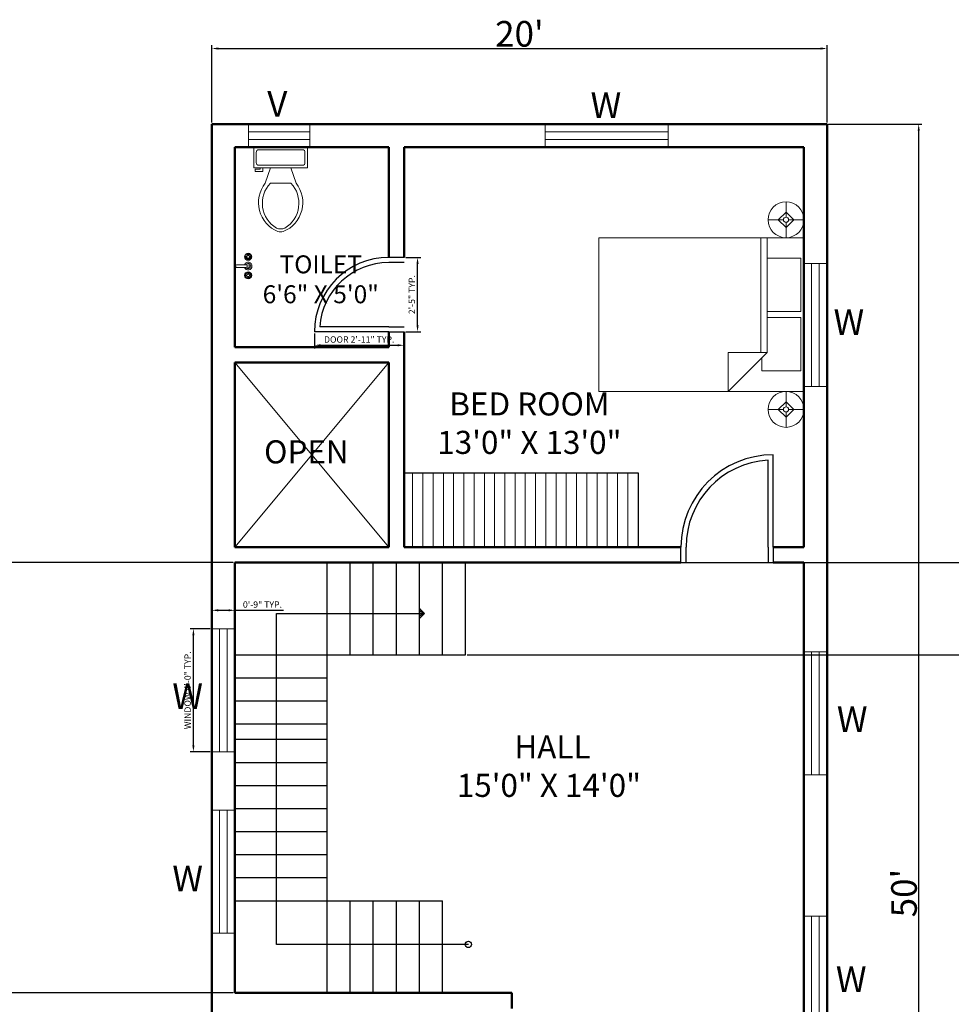
# Model space of a CAD drawing. Units: inches. Extents: x 995 to 2141, y 2161 to 2928.
# Tile 5 of 7: x 1358 to 1721, y 2537 to 2921. Entities that reach past the tile are written whole.
import ezdxf

# ---------------------------------------------------------------- set-up
doc = ezdxf.new("R2010")
doc.units = ezdxf.units.IN
for name, color, linetype, lineweight in [('A-ANNO-DIMS', 2, 'Continuous', 18), ('A-ANNO-TEXT', 7, 'Continuous', 18), ('A-AREA-IDEN', 7, 'Continuous', 25), ('A-DOOR', 3, 'Continuous', 25), ('A-FLOR-CASE', 8, 'Continuous', 25), ('A-FLOR-CASE-PATT', 252, 'Continuous', 13), ('A-FLOR-FIXT', 9, 'Continuous', 18), ('A-FLOR-OPEN', 8, 'Continuous', 13), ('A-FLOR-STRS', 7, 'Continuous', 25), ('A-FURN', 8, 'Continuous', 18), ('A-GLAZ', 4, 'Continuous', 18), ('A-WALL', 7, 'Continuous', 50)]:
    doc.layers.add(name, color=color, linetype=linetype, lineweight=lineweight)
doc.styles.get("Standard").update_dxf_attribs({"font": 'arial.ttf'})
doc.dimstyles.new('ISO-25', dxfattribs={"dimtxt": 2.5, "dimasz": 2.5, "dimexe": 1.25, "dimexo": 0.625, "dimtad": 1, "dimdec": 0, "dimlunit": 3, "dimtxsty": 'Standard', "dimcen": 2.5, "dimadec": 0, "dimazin": 0, "dimtfac": 1, "dimtdec": 0, "dimtmove": 0, "dimatfit": 3, "dimfxl": 1, "dimarcsym": 0})

# ---------------------------------------------------------------- blocks, each defined once
blk = doc.blocks.new('Bed - Queen')
for p, q in [((0, -80.00003), (0, 0)), ((0, 0), (59.99999, 0)), ((59.99999, 0), (59.99999, -80.00003)), ((7.99999, -1.2), (28.79998, -1.2)), ((7.99999, -14.4), (7.99999, -1.2)), ((28.79998, -1.2), (28.79998, -14.4)), ((31.19999, -1.2), (51.99999, -1.2)), ((31.19999, -14.4), (31.19999, -1.2)), ((51.99999, -1.2), (51.99999, -16.4)), ((0, -14.4), (44.8, -14.4)), ((59.99999, -29.6), (44.8, -14.4)), ((44.8, -14.4), (44.8, -29.6)), ((44.8, -16.8), (0, -16.8)), ((51.99999, -16.4), (46.79936, -16.4)), ((44.8, -29.6), (59.99999, -29.6)), ((59.99999, -80.00003), (0, -80.00003))]:
    blk.add_line(p, q)
blk = doc.blocks.new('Lamp - Table')
for p, q in [((0, 7), (0, 1)), ((-1, 0), (-7, 0)), ((0, 3), (-3, 0)), ((-3, 0), (0, -3)), ((3, 0), (0, 3)), ((0, -3), (3, 0)), ((1, 0), (7, 0)), ((0, -1), (0, -7))]:
    blk.add_line(p, q)
for radius in [7, 1]:
    blk.add_circle((0, 0), radius)
blk = doc.blocks.new('Toilet - top')
for p, q in [((9.5, -6), (9.5, -2)), ((-10, -8.5), (-8, -8.5)), ((-10, -9.5), (-10, -8.5)), ((-7, -9.5), (-10, -9.5)), ((-8, -8.5), (-8, -8)), ((-7, -8), (-7, -9.5)), ((-4, -8), (-6, -14)), ((4, -8), (6, -14)), ((4, -14), (-4, -14))]:
    blk.add_line(p, q)
blk.add_lwpolyline([(10.5, -8), (10.5, 0), (-10.5, 0), (-10.5, -8)], close=True)
for points in [[(-9.5, -2), (-9.5, -6)], [(8.5, -1), (-8.5, -1)], [(-8.5, -7), (8.5, -7)]]:
    blk.add_lwpolyline(points)
for centre, radius, start, end in [((-8.62, -1.88), 0.884, 81.8699, 188.1301), ((8.62, -1.88), 0.884, 351.8699, 98.1301), ((-8.62, -6.12), 0.884, 171.8699, 278.1301), ((8.62, -6.12), 0.884, 261.8699, 8.1301), ((3.52, -21.58), 12.17, 141.4691, 247.9714), ((4.2, -21.82), 11.33, 136.3677, 238.9468), ((-3.52, -21.58), 12.17, 292.0284, 38.5307), ((-4.2, -21.82), 11.33, 301.053, 43.6321), ((0, -27.88), 4, 245.7318, 294.2682), ((0, -29), 4, 254.8605, 285.1395)]:
    blk.add_arc(centre, radius, start, end)
blk = doc.blocks.new('Faucet - Bathroom top')
for p, q in [((-4.107, 0.125), (-4.375, 0.125)), ((-3.75, 0.4788), (-3.75, 0.75)), ((-3.5, 0.482), (-3.5, 0.75)), ((-3.1461, 0.125), (-2.875, 0.125)), ((3.143, 0.125), (2.875, 0.125)), ((3.5, 0.4788), (3.5, 0.75)), ((3.75, 0.482), (3.75, 0.75)), ((4.1039, 0.125), (4.375, 0.125)), ((-4.1039, -0.125), (-4.375, -0.125)), ((-3.75, -0.4821), (-3.75, -0.75)), ((-3.5, -0.4789), (-3.5, -0.75)), ((-3.143, -0.125), (-2.875, -0.125)), ((-0.5, -0.8639), (-0.5, -4.5)), ((0.5, -4.5), (0.5, -0.8631)), ((3.1461, -0.125), (2.875, -0.125)), ((3.5, -0.4821), (3.5, -0.75)), ((3.75, -0.4789), (3.75, -0.75)), ((4.107, -0.125), (4.375, -0.125))]:
    blk.add_line(p, q)
for centre, radius in [((-3.625, 0), 1.375), ((-4.625, 0), 0.2795), ((-3.625, 0), 0.5), ((-3.625, 1), 0.2795), ((-2.625, 0), 0.2795), ((0, 0), 0.5), ((3.625, 0), 1.375), ((2.625, 0), 0.2795), ((3.625, 0), 0.5), ((3.625, 1), 0.2795), ((4.625, 0), 0.2795), ((-3.625, -1), 0.2795), ((3.625, -1), 0.2795)]:
    blk.add_circle(centre, radius)
for centre, radius, start, end in [((-3.625, 0), 1, 105.2407, 164.2093), ((-3.625, 0), 1, 16.44125, 74.07887), ((0, 0), 1.5, 289.6514, 250.3603), ((0, 0), 1, 300.3431, 239.7554), ((3.625, 0), 1, 106.12, 164.0884), ((3.625, 0), 1, 16.23422, 73.90469), ((-3.625, 0), 1, 196.2342, 253.9047), ((-3.625, 0), 1, 286.12, 344.0884), ((3.625, 0), 1, 196.4413, 254.0789), ((3.625, 0), 1, 285.2407, 344.2093), ((0, -4.5), 0.5, 180, 0)]:
    blk.add_arc(centre, radius, start, end)
blk = doc.blocks.new('*D18')
at = {"layer": 'A-ANNO-DIMS', "color": 0, "lineweight": -2, "transparency": 16777216}
for p, q in [((1433, 2881.14), (1433, 2911.31)), ((1435.5, 2910.06), (1670.5, 2910.06)), ((1673, 2881.14), (1673, 2911.31))]:
    blk.add_line(p, q, dxfattribs=at)
at = {"layer": 'A-ANNO-DIMS', "color": 0, "transparency": 16777216}
for points in [[(1435.5, 2910.48), (1435.5, 2909.64), (1433, 2910.06)], [(1670.5, 2910.48), (1670.5, 2909.64), (1673, 2910.06)]]:
    blk.add_solid(points, dxfattribs=at)
at = {"layer": 'Defpoints', "color": 0, "transparency": 16777216}
for p in [(1673, 2910.06), (1433, 2880.52), (1673, 2880.52)]:
    blk.add_point(p, dxfattribs=at)
at = {"layer": 'A-ANNO-DIMS', "color": 0, "transparency": 16777216, "insert": (1553, 2915.79), "char_height": 2.5, "attachment_point": 5}
blk.add_mtext("{\\H4x;20'}", dxfattribs=at)
blk = doc.blocks.new('*D21')
at = {"layer": 'A-ANNO-DIMS', "color": 0, "lineweight": -2, "transparency": 16777216}
for p, q in [((1673.63, 2880.52), (1710.02, 2880.52)), ((1708.77, 2283.02), (1708.77, 2878.02)), ((1673.63, 2280.52), (1710.02, 2280.52))]:
    blk.add_line(p, q, dxfattribs=at)
at = {"layer": 'A-ANNO-DIMS', "color": 0, "transparency": 16777216}
for points in [[(1708.36, 2878.02), (1709.19, 2878.02), (1708.77, 2880.52)], [(1708.36, 2283.02), (1709.19, 2283.02), (1708.77, 2280.52)]]:
    blk.add_solid(points, dxfattribs=at)
at = {"layer": 'Defpoints', "color": 0, "transparency": 16777216}
for p in [(1673, 2880.52), (1708.77, 2880.52), (1673, 2280.52)]:
    blk.add_point(p, dxfattribs=at)
at = {"layer": 'A-ANNO-DIMS', "color": 0, "transparency": 16777216, "insert": (1703.04, 2580.52), "char_height": 2.5, "attachment_point": 5, "rotation": 90}
blk.add_mtext("{\\H4x;50'}", dxfattribs=at)
blk = doc.blocks.new('WIN-48IN')
for p, q in [((0, 48), (0, 0)), ((9, 48), (0, 48)), ((3, 48), (3, 0)), ((6, 0), (6, 48)), ((9, 0), (9, 48)), ((0, 0), (9, 0))]:
    blk.add_line(p, q)
blk = doc.blocks.new('VENT-24IN')
for p, q in [((24, 9), (0, 9)), ((0, 9), (0, 0)), ((24, 9), (24, 0)), ((24, 6), (0, 6)), ((0, 3), (24, 3)), ((0, 0), (24, 0))]:
    blk.add_line(p, q)
blk = doc.blocks.new('DOOR-29IN-6IN-JAMB')
for p, q in [((35, 29), (29, 29)), ((35, 27), (29, 27)), ((29, 0), (0, 0)), ((29, 2), (2.07, 2)), ((29, 2), (35, 2)), ((29, 0), (35, 0))]:
    blk.add_line(p, q)
for radius, end in [(29, 180), (27, 175.752)]:
    blk.add_arc((29, 0), radius, 90, end)
blk = doc.blocks.new('DOOR-36IN-SWING')
for p, q in [((36, 0), (36, 36)), ((34, 0), (34, 33.94))]:
    blk.add_line(p, q)
for radius, start in [(36, 90), (34, 93.3723)]:
    blk.add_arc((36, 0), radius, start, 180)
blk = doc.blocks.new('OPENING-CROSS-60X72')
for p, q in [((60, 72), (0, 0)), ((0, 72), (60, 0))]:
    blk.add_line(p, q)
blk = doc.blocks.new('*D28')
at = {"layer": 'A-ANNO-DIMS', "color": 0, "lineweight": -2, "transparency": 16777216}
for p, q in [((1432.38, 2683.64), (1424.55, 2683.64)), ((1425.8, 2638.14), (1425.8, 2681.14)), ((1432.38, 2635.64), (1424.55, 2635.64))]:
    blk.add_line(p, q, dxfattribs=at)
at = {"layer": 'A-ANNO-DIMS', "color": 0, "transparency": 16777216}
for points in [[(1425.39, 2681.14), (1426.22, 2681.14), (1425.8, 2683.64)], [(1425.39, 2638.14), (1426.22, 2638.14), (1425.8, 2635.64)]]:
    blk.add_solid(points, dxfattribs=at)
at = {"layer": 'Defpoints', "color": 0, "transparency": 16777216}
for p in [(1425.8, 2683.64), (1433, 2683.64), (1433, 2635.64)]:
    blk.add_point(p, dxfattribs=at)
at = {"layer": 'A-ANNO-DIMS', "color": 0, "transparency": 16777216, "insert": (1423.88, 2659.64), "char_height": 2.5, "attachment_point": 5, "rotation": 90}
blk.add_mtext('WINDOW 4\'-0" TYP.', dxfattribs=at)
blk = doc.blocks.new('*D29')
at = {"layer": 'A-ANNO-DIMS', "color": 0, "lineweight": -2, "transparency": 16777216}
for p, q in [((1433, 2684.27), (1433, 2692.09)), ((1435.5, 2690.84), (1439.5, 2690.84)), ((1442, 2684.27), (1442, 2692.09)), ((1442, 2690.84), (1460.99, 2690.84))]:
    blk.add_line(p, q, dxfattribs=at)
at = {"layer": 'A-ANNO-DIMS', "color": 0, "transparency": 16777216}
for points in [[(1435.5, 2691.26), (1435.5, 2690.43), (1433, 2690.84)], [(1439.5, 2691.26), (1439.5, 2690.43), (1442, 2690.84)]]:
    blk.add_solid(points, dxfattribs=at)
at = {"layer": 'Defpoints', "color": 0, "transparency": 16777216}
for p in [(1442, 2690.84), (1433, 2683.64), (1442, 2683.64)]:
    blk.add_point(p, dxfattribs=at)
at = {"layer": 'A-ANNO-DIMS', "color": 0, "transparency": 16777216, "insert": (1452.75, 2692.75), "char_height": 2.5, "attachment_point": 5}
blk.add_mtext('0\'-9" TYP.', dxfattribs=at)
blk = doc.blocks.new('*D36')
at = {"layer": 'A-ANNO-DIMS', "color": 0, "lineweight": -2, "transparency": 16777216}
for p, q in [((1473, 2798.89), (1473, 2793.02)), ((1508, 2798.89), (1508, 2793.02)), ((1475.5, 2794.27), (1505.5, 2794.27))]:
    blk.add_line(p, q, dxfattribs=at)
at = {"layer": 'A-ANNO-DIMS', "color": 0, "transparency": 16777216}
for points in [[(1475.5, 2794.68), (1475.5, 2793.85), (1473, 2794.27)], [(1505.5, 2794.68), (1505.5, 2793.85), (1508, 2794.27)]]:
    blk.add_solid(points, dxfattribs=at)
at = {"layer": 'Defpoints', "color": 0, "transparency": 16777216}
for p in [(1473, 2799.52), (1508, 2799.52), (1508, 2794.27)]:
    blk.add_point(p, dxfattribs=at)
at = {"layer": 'A-ANNO-DIMS', "color": 0, "transparency": 16777216, "insert": (1490.5, 2796.19), "char_height": 2.5, "attachment_point": 5}
blk.add_mtext('DOOR 2\'-11" TYP.', dxfattribs=at)
blk = doc.blocks.new('*D37')
at = {"layer": 'A-ANNO-DIMS', "color": 0, "lineweight": -2, "transparency": 16777216}
for p, q in [((1508.63, 2828.52), (1514.5, 2828.52)), ((1513.25, 2802.02), (1513.25, 2826.02)), ((1508.63, 2799.52), (1514.5, 2799.52))]:
    blk.add_line(p, q, dxfattribs=at)
at = {"layer": 'A-ANNO-DIMS', "color": 0, "transparency": 16777216}
for points in [[(1512.84, 2826.02), (1513.67, 2826.02), (1513.25, 2828.52)], [(1512.84, 2802.02), (1513.67, 2802.02), (1513.25, 2799.52)]]:
    blk.add_solid(points, dxfattribs=at)
at = {"layer": 'Defpoints', "color": 0, "transparency": 16777216}
for p in [(1508, 2828.52), (1513.25, 2828.52), (1508, 2799.52)]:
    blk.add_point(p, dxfattribs=at)
at = {"layer": 'A-ANNO-DIMS', "color": 0, "transparency": 16777216, "insert": (1511.35, 2814.02), "char_height": 2.5, "attachment_point": 5, "rotation": 90}
blk.add_mtext('2\'-5" TYP.', dxfattribs=at)
blk = doc.blocks.new('*D64')
at = {"layer": 'A-ANNO-DIMS', "color": 0, "lineweight": -2, "transparency": 16777216}
for p, q in [((1532.63, 2709.52), (2141.3, 2709.52)), ((2140.05, 2676.02), (2140.05, 2707.02)), ((1532.63, 2673.52), (2141.3, 2673.52))]:
    blk.add_line(p, q, dxfattribs=at)
at = {"layer": 'A-ANNO-DIMS', "color": 0, "transparency": 16777216}
for points in [[(2139.63, 2707.02), (2140.46, 2707.02), (2140.05, 2709.52)], [(2139.63, 2676.02), (2140.46, 2676.02), (2140.05, 2673.52)]]:
    blk.add_solid(points, dxfattribs=at)
at = {"layer": 'Defpoints', "color": 0, "transparency": 16777216}
for p in [(1532, 2709.52), (2140.05, 2709.52), (1532, 2673.52)]:
    blk.add_point(p, dxfattribs=at)
at = {"layer": 'A-ANNO-DIMS', "color": 0, "transparency": 16777216, "insert": (2138.14, 2691.52), "char_height": 2.5, "attachment_point": 5, "rotation": 90}
blk.add_mtext('3\'-0"', dxfattribs=at)
blk = doc.blocks.new('*D65')
at = {"layer": 'A-ANNO-DIMS', "color": 0, "lineweight": -2, "transparency": 16777216}
for p, q in [((1441.38, 2709.52), (996.93, 2709.52)), ((998.18, 2544.02), (998.18, 2707.02)), ((1441.38, 2541.52), (996.93, 2541.52))]:
    blk.add_line(p, q, dxfattribs=at)
at = {"layer": 'A-ANNO-DIMS', "color": 0, "transparency": 16777216}
for points in [[(997.77, 2707.02), (998.6, 2707.02), (998.18, 2709.52)], [(997.77, 2544.02), (998.6, 2544.02), (998.18, 2541.52)]]:
    blk.add_solid(points, dxfattribs=at)
at = {"layer": 'Defpoints', "color": 0, "transparency": 16777216}
for p in [(998.18, 2709.52), (1442, 2709.52), (1442, 2541.52)]:
    blk.add_point(p, dxfattribs=at)
at = {"layer": 'A-ANNO-DIMS', "color": 0, "transparency": 16777216, "insert": (996.28, 2625.52), "char_height": 2.5, "attachment_point": 5, "rotation": 90}
blk.add_mtext('14\'-0"', dxfattribs=at)

msp = doc.modelspace()

# ---------------------------------------------------------------- hatches: boundary and pattern name
at = {"layer": 'A-FLOR-CASE-PATT'}
h = msp.add_hatch(dxfattribs=at)
h.set_pattern_fill('ANSI31', color=256, scale=1.259274, angle=45, style=0)
h.paths.add_polyline_path([(1509.3, 2715.52), (1597.3, 2715.52), (1597.3, 2744.52), (1509.3, 2744.52)])

# ---------------------------------------------------------------- linework, layer by layer
at = {"layer": 'A-DOOR'}
for p, q in [((1616, 2709.52), (1616, 2715.52)), ((1618, 2709.52), (1618, 2715.52)), ((1650, 2715.52), (1650, 2709.52)), ((1652, 2715.52), (1652, 2709.52))]:
    msp.add_line(p, q, dxfattribs=at)
at = {"layer": 'A-FLOR-CASE'}
for p, q in [((1508, 2744.52), (1599.3, 2744.52)), ((1599.3, 2744.52), (1599.3, 2715.52))]:
    msp.add_line(p, q, dxfattribs=at)
at = {"layer": 'A-FLOR-STRS'}
for p, q in [((1478, 2541.52), (1478, 2709.52)), ((1487, 2673.52), (1487, 2709.52)), ((1496, 2673.52), (1496, 2709.52)), ((1505, 2673.52), (1505, 2709.52)), ((1514, 2673.52), (1514, 2709.52)), ((1523, 2673.52), (1523, 2709.52)), ((1532, 2673.52), (1532, 2709.52)), ((1458.26, 2560.49), (1458.26, 2689.66)), ((1458.26, 2689.66), (1514, 2689.66)), ((1514, 2689.66), (1514, 2691.66)), ((1514, 2691.66), (1514, 2689.66)), ((1516, 2689.66), (1514, 2691.52)), ((1514, 2691.52), (1516, 2689.66)), ((1516, 2689.66), (1514, 2690.66)), ((1514, 2689.66), (1514, 2687.66)), ((1514, 2687.66), (1514, 2689.66)), ((1514, 2689.66), (1516, 2689.66)), ((1516, 2689.66), (1514, 2689.66)), ((1514, 2689.66), (1514, 2689.66)), ((1514, 2689.66), (1516, 2689.66)), ((1516, 2689.66), (1514, 2687.66)), ((1514, 2688.66), (1516, 2689.66)), ((1514, 2687.66), (1514, 2688.66)), ((1442, 2673.52), (1532, 2673.52)), ((1442, 2664.52), (1478, 2664.52)), ((1442, 2655.52), (1478, 2655.52)), ((1442, 2646.52), (1478, 2646.52)), ((1442, 2640.52), (1478, 2640.52)), ((1442, 2631.52), (1478, 2631.52)), ((1442, 2622.52), (1478, 2622.52)), ((1442, 2613.52), (1478, 2613.52)), ((1442, 2604.52), (1478, 2604.52)), ((1442, 2595.52), (1478, 2595.52)), ((1442, 2586.52), (1478, 2586.52)), ((1442, 2577.52), (1523, 2577.52)), ((1487, 2541.52), (1487, 2577.52)), ((1496, 2541.52), (1496, 2577.52)), ((1505, 2541.52), (1505, 2577.52)), ((1514, 2541.52), (1514, 2577.52)), ((1523, 2541.52), (1523, 2577.52)), ((1533.07, 2560.49), (1458.26, 2560.49))]:
    msp.add_line(p, q, dxfattribs=at)
msp.add_circle((1533.07, 2560.49), 1.26, dxfattribs=at)
at = {"layer": 'A-WALL'}
for p, q in [((1433, 2880.52), (1673, 2880.52)), ((1433, 2280.52), (1433, 2880.52)), ((1673, 2880.52), (1673, 2280.52)), ((1442, 2871.52), (1502, 2871.52)), ((1442, 2793.52), (1442, 2871.52)), ((1502, 2871.52), (1502, 2828.52)), ((1508, 2871.52), (1508, 2828.52)), ((1508, 2871.52), (1664, 2871.52)), ((1664, 2871.52), (1664, 2715.52)), ((1502, 2793.52), (1502, 2799.52)), ((1502, 2799.52), (1502, 2793.52)), ((1508, 2799.52), (1508, 2715.52)), ((1442, 2793.52), (1448, 2793.52)), ((1472, 2793.52), (1448, 2793.52)), ((1472, 2793.52), (1502, 2793.52)), ((1442, 2715.52), (1442, 2787.52)), ((1442, 2787.52), (1448, 2787.52)), ((1442, 2787.52), (1448, 2787.52)), ((1442, 2715.52), (1442, 2787.52)), ((1448, 2787.52), (1472, 2787.52)), ((1472, 2787.52), (1502, 2787.52)), ((1502, 2787.52), (1502, 2715.52)), ((1442, 2715.52), (1502, 2715.52)), ((1508, 2715.52), (1616, 2715.52)), ((1664, 2715.52), (1652, 2715.52)), ((1652, 2715.52), (1664, 2715.52)), ((1442, 2709.52), (1616, 2709.52)), ((1442, 2541.52), (1442, 2709.52)), ((1652, 2709.52), (1664, 2709.52)), ((1664, 2709.52), (1664, 2483.52)), ((1442, 2541.52), (1550, 2541.52)), ((1550, 2535.52), (1550, 2541.52))]:
    msp.add_line(p, q, dxfattribs=at)

# ---------------------------------------------------------------- block references
at = {"layer": 'A-DOOR'}
for name, p in [('DOOR-29IN-6IN-JAMB', (1473, 2799.52)), ('DOOR-36IN-SWING', (1616, 2715.52))]:
    msp.add_blockref(name, p, dxfattribs=at)
at = {"layer": 'A-FLOR-FIXT'}
msp.add_blockref('Toilet - top', (1459.84, 2871.52), dxfattribs=at)
at = {"layer": 'A-FLOR-FIXT', "rotation": 270}
msp.add_blockref('Faucet - Bathroom top', (1447.16, 2825.17), dxfattribs=at)
at = {"layer": 'A-FLOR-OPEN'}
msp.add_blockref('OPENING-CROSS-60X72', (1442, 2715.52), dxfattribs=at)
at = {"layer": 'A-FURN', "rotation": 270}
for name, p in [('Lamp - Table', (1657, 2843.24)), ('Bed - Queen', (1664, 2836.24)), ('Lamp - Table', (1657, 2769.24))]:
    msp.add_blockref(name, p, dxfattribs=at)
at = {"layer": 'A-GLAZ'}
for name, p, rotation in [('VENT-24IN', (1471.29, 2880.52), 180), ('WIN-48IN', (1611.02, 2871.52), 90.00000000000104)]:
    msp.add_blockref(name, p, dxfattribs=dict(at, rotation=rotation))
for p in [(1664, 2778.21), (1433, 2635.64), (1664, 2626.67), (1433, 2564.91), (1664, 2523.48)]:
    msp.add_blockref('WIN-48IN', p, dxfattribs=at)

# ---------------------------------------------------------------- texts
at = {"layer": 'A-ANNO-TEXT', "char_height": 10, "attachment_point": 1}
for s, insert in [('V', (1454.61, 2893.46)), ('W', (1580.75, 2892.93)), ('W', (1675.54, 2808.33)), ('W', (1417.57, 2662.32)), ('W', (1676.84, 2653.36)), ('W', (1417.57, 2591.25)), ('W', (1676.45, 2551.88))]:
    msp.add_mtext_dynamic_manual_height_columns(s, width=112.484, gutter_width=12.5, heights=[0], dxfattribs=dict(at, insert=insert))
at = {"layer": 'A-AREA-IDEN', "attachment_point": 1}
for s, width, insert, char_height in [('\\pxqc;TOILET\\P6\'6" X 5\'0"', 53.0246, (1448.98, 2829.34), 7), ('\\pxqc;BED ROOM ^J13\'0" X 13\'0"', 109.7687, (1502, 2775.87), 9), ('\\pxqc;OPEN ', 52.2467, (1443.76, 2757.18), 9), ('\\pxqc; HALL \\P15\'0" X 14\'0"', 103.3264, (1512.84, 2642.04), 9)]:
    msp.add_mtext_dynamic_manual_height_columns(s, width=width, gutter_width=12.5, heights=[0], dxfattribs=dict(at, insert=insert, char_height=char_height))

# ---------------------------------------------------------------- dimensions: what is measured, and where the dimension line sits
at = {"layer": 'A-ANNO-DIMS'}
for base, p1, p2, text, override, picture, middle in [((1673, 2910.06), (1433, 2880.52), (1673, 2880.52), "{\\H4x;20'}", {"dimclrd": 0, "dimclre": 0, "dimclrt": 0}, '*D18', (1553, 2915.79)), ((1508, 2794.27), (1473, 2799.52), (1508, 2799.52), 'DOOR <> TYP.', {"dimdec": 1, "dimlfac": 1, "dimrnd": 0, "dimzin": 1, "dimdsep": 46, "dimlunit": 4, "dimfrac": 2}, '*D36', (1490.5, 2796.19)), ((1442, 2690.84), (1433, 2683.64), (1442, 2683.64), '<> TYP.', {"dimdec": 1, "dimlfac": 1, "dimrnd": 0, "dimzin": 1, "dimdsep": 46, "dimlunit": 4, "dimfrac": 2}, '*D29', (1452.75, 2692.75))]:
    dim = msp.add_linear_dim(base=base, p1=p1, p2=p2, text=text, dimstyle='ISO-25', override=override, dxfattribs=at)
    dim.commit()
    dim.dimension.update_dxf_attribs({"geometry": picture, "text_midpoint": middle})
for base, p1, p2, text, override, picture, middle in [((1708.77, 2880.52), (1673, 2280.52), (1673, 2880.52), "{\\H4x;50'}", {"dimclrd": 0, "dimclre": 0, "dimclrt": 0}, '*D21', (1703.04, 2580.52)), ((1513.25, 2828.52), (1508, 2799.52), (1508, 2828.52), '<> TYP.', {"dimdec": 1, "dimlfac": 1, "dimrnd": 0, "dimzin": 1, "dimdsep": 46, "dimlunit": 4, "dimfrac": 2}, '*D37', (1511.35, 2814.02)), ((1425.8, 2683.64), (1433, 2635.64), (1433, 2683.64), 'WINDOW <> TYP.', {"dimdec": 1, "dimlfac": 1, "dimrnd": 0, "dimzin": 1, "dimdsep": 46, "dimlunit": 4, "dimfrac": 2}, '*D28', (1423.88, 2659.64))]:
    dim = msp.add_linear_dim(base=base, p1=p1, p2=p2, angle=90, text=text, dimstyle='ISO-25', override=override, dxfattribs=at)
    dim.commit()
    dim.dimension.update_dxf_attribs({"geometry": picture, "text_midpoint": middle})
for base, p1, p2, picture, middle in [((998.18, 2709.52), (1442, 2541.52), (1442, 2709.52), '*D65', (996.28, 2625.52)), ((2140.05, 2709.52), (1532, 2673.52), (1532, 2709.52), '*D64', (2138.14, 2691.52))]:
    dim = msp.add_linear_dim(base=base, p1=p1, p2=p2, angle=90, dimstyle='ISO-25', override={"dimdec": 1, "dimlfac": 1, "dimrnd": 0, "dimzin": 1, "dimdsep": 46, "dimlunit": 4, "dimfrac": 2}, dxfattribs=at)
    dim.commit()
    dim.dimension.update_dxf_attribs({"geometry": picture, "text_midpoint": middle})

doc.saveas('drawing.dxf')
